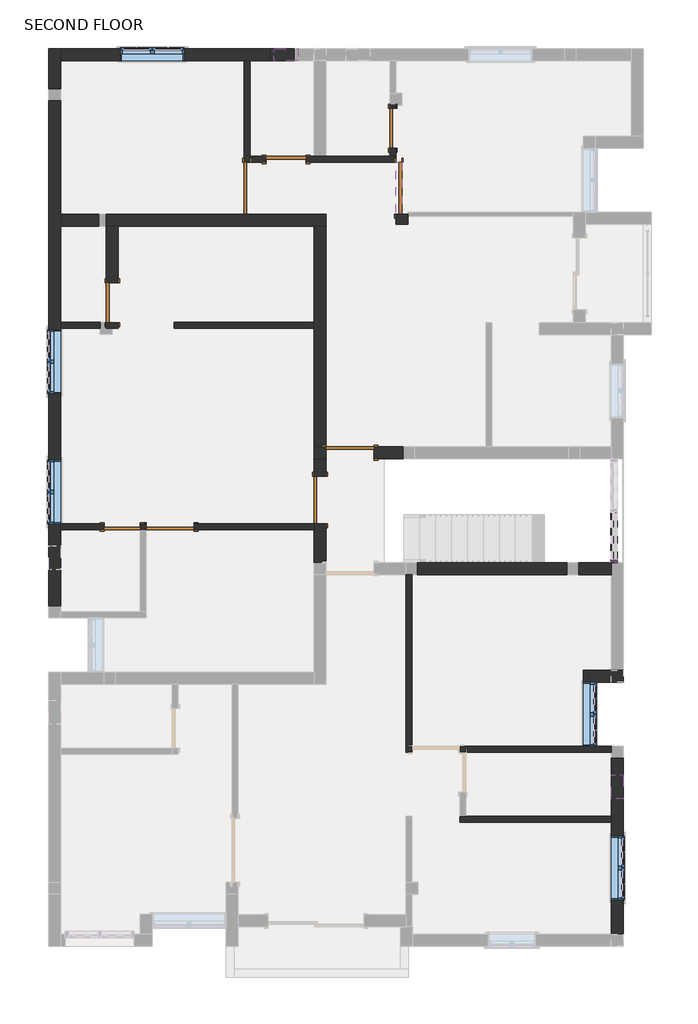
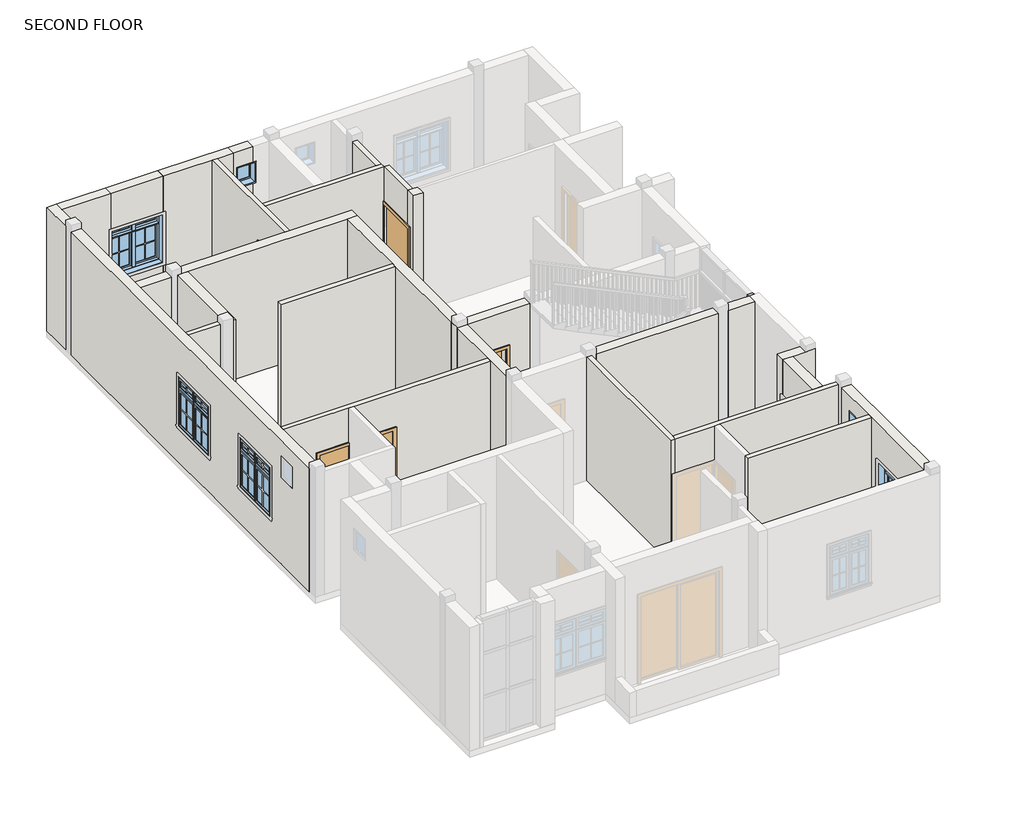
# One storey, part 2 of 6: 29 walls, 9 doors, 7 windows, 3 members.
"""IFC4 building model written with IfcOpenShell, lengths in millimetres."""

from ifc_helpers import new_model, si_unit, frame, origin, place, context, project, spatial, polyline, outline, extrude, faceted_brep, transform, mapped, element, save
from components import door_64f31108, door_78caadf7, door_214872d5, door_bb98abfd, door_43e5c869, door_0217d254, single_flush_3_x7_a90ba1ad, single_flush_3_x7_e5f9f3c4, member_f1f71bde, member_00c01c4d, member_ecafcbb3, window_abb441dd, window_casement_double_awning_double_4_x4_dd9041c6

model = new_model("IFC4")

# Units and contexts
model_context = context("Model", 3, world=origin())
ifc_project = project(units=[si_unit("LENGTHUNIT", "METRE", prefix="MILLI")], contexts=[model_context])

# Site, building, storey
site = spatial("IfcSite", under=ifc_project)
building = spatial("IfcBuilding", under=site)
storey = spatial("IfcBuildingStorey", under=building, Name="SECOND FLOOR", Elevation=6400.8)

# Doors
placement = place(None, origin())
door_shape = door_64f31108(model_context)
element("IfcDoor", 1, ObjectType="Single-Flush : 2'3\"X7'", at=placement, inside=storey, context=model_context, shape_type="MappedRepresentation", body=[
    mapped(door_shape, transform((-5358.7865981, 175.2287587, 6400.8), x_axis=(1.0, 0.0, 0.0), y_axis=(0.0, 1.0, 0.0), z_axis=(0.0, 0.0, 1.0))),
])
door_2_shape = door_78caadf7(model_context)
element("IfcDoor", 2, ObjectType="Single-Flush : 2'6\"X7'", at=placement, inside=storey, context=model_context, shape_type="MappedRepresentation", body=[
    mapped(door_2_shape, transform((-196.2365981, 7776.1787587, 6400.8), x_axis=(0.0, -1.0, 0.0), y_axis=(1.0, 0.0, 0.0), z_axis=(0.0, 0.0, 1.0))),
])
door_3_shape = door_214872d5(model_context)
element("IfcDoor", 3, ObjectType="Single-Flush : 2'6\"X7'", at=placement, inside=storey, context=model_context, shape_type="MappedRepresentation", body=[
    mapped(door_3_shape, transform((-2234.5865981, 7185.6287587, 6400.8), x_axis=(1.0, 0.0, 0.0), y_axis=(0.0, 1.0, 0.0), z_axis=(0.0, 0.0, 1.0))),
])
door_4_shape = door_bb98abfd(model_context)
element("IfcDoor", 4, ObjectType="Single-Flush : 2'6\"X7'", at=placement, inside=storey, context=model_context, shape_type="MappedRepresentation", body=[
    mapped(door_4_shape, transform((-5549.2865981, 4455.1287587, 6400.8), x_axis=(0.0, 1.0, 0.0), y_axis=(-1.0, 0.0, 0.0), z_axis=(0.0, 0.0, 1.0))),
])
door_5_shape = door_43e5c869(model_context)
element("IfcDoor", 5, ObjectType="Single-Flush : 3'3\"X7'", at=placement, inside=storey, context=model_context, shape_type="MappedRepresentation", body=[
    mapped(door_5_shape, transform((-2977.5365981, 6633.1787587, 6400.8), x_axis=(0.0, -1.0, 0.0), y_axis=(1.0, 0.0, 0.0), z_axis=(0.0, 0.0, 1.0))),
])
door_6_shape = door_0217d254(model_context)
element("IfcDoor", 6, ObjectType="Single-Flush : 3'3\"X7'", at=placement, inside=storey, context=model_context, shape_type="MappedRepresentation", body=[
    mapped(door_6_shape, transform((-81.9365981, 6633.1787587, 6400.8), x_axis=(0.0, -1.0, 0.0), y_axis=(1.0, 0.0, 0.0), z_axis=(0.0, 0.0, 1.0))),
])
single_flush_3_x7_shape = single_flush_3_x7_a90ba1ad(model_context)
element("IfcDoor", 7, ObjectType="Single-Flush : 3'X7'", at=placement, inside=storey, context=model_context, shape_type="MappedRepresentation", body=[
    mapped(single_flush_3_x7_shape, transform((-1586.8865981, 689.5787587, 6400.8), x_axis=(0.0, -1.0, 0.0), y_axis=(1.0, 0.0, 0.0), z_axis=(0.0, 0.0, 1.0))),
])
element("IfcDoor", 8, ObjectType="Single-Flush : 3'X7'", at=placement, inside=storey, context=model_context, shape_type="MappedRepresentation", body=[
    mapped(single_flush_3_x7_shape, transform((-1015.3865981, 1591.2787587, 6400.8), x_axis=(-1.0, 0.0, 0.0), y_axis=(0.0, -1.0, 0.0), z_axis=(0.0, 0.0, 1.0))),
])
single_flush_3_x7_2_shape = single_flush_3_x7_e5f9f3c4(model_context)
element("IfcDoor", 9, ObjectType="Single-Flush : 3'X7'", at=placement, inside=storey, context=model_context, shape_type="MappedRepresentation", body=[
    mapped(single_flush_3_x7_2_shape, transform((-4444.3865981, 175.2287587, 6400.8), x_axis=(-1.0, 0.0, 0.0), y_axis=(0.0, -1.0, 0.0), z_axis=(0.0, 0.0, 1.0))),
])

# Members
member_shape = member_f1f71bde(model_context)
element("IfcMember", 10, ObjectType="Rectangular Mullion : 2.5\" x 5\" rectangular", at=placement, inside=storey, context=model_context, shape_type="MappedRepresentation", body=[
    mapped(member_shape, transform((4026.5134019, -440.7212413, 6400.8), x_axis=(0.0, 0.0, -1.0), y_axis=(1.0, 0.0, 0.0), z_axis=(0.0, -1.0, 0.0))),
])
member_2_shape = member_00c01c4d(model_context)
element("IfcMember", 11, ObjectType="Rectangular Mullion : 2.5\" x 5\" rectangular", at=placement, inside=storey, context=model_context, shape_type="MappedRepresentation", body=[
    mapped(member_2_shape, transform((4026.5134019, -504.2212413, 7956.55), x_axis=(0.0, -1.0, 0.0), y_axis=(1.0, 0.0, 0.0), z_axis=(0.0, 0.0, 1.0))),
])
member_3_shape = member_ecafcbb3(model_context)
element("IfcMember", 12, ObjectType="Rectangular Mullion : 2.5\" x 5\" rectangular", at=placement, inside=storey, context=model_context, shape_type="MappedRepresentation", body=[
    mapped(member_3_shape, transform((4026.5134019, -504.2212413, 9448.8), x_axis=(0.0, -1.0, 0.0), y_axis=(1.0, 0.0, 0.0), z_axis=(0.0, 0.0, 1.0))),
])

# Walls
element("IfcWall", 13, ObjectType="4.5\"", at=placement, inside=storey, context=model_context, shape_type="Brep", body=[
    faceted_brep([(-3034.6865981, 6137.8787587, 9448.8), (-3034.6865981, 9071.5787587, 9448.8), (-3034.6865981, 9071.5787587, 6400.8), (-3034.6865981, 7128.4787587, 6400.8), (-3034.6865981, 7128.4787587, 8534.4), (-3034.6865981, 6137.8787587, 8534.4), (-2920.3865981, 9071.5787587, 9448.8), (-2920.3865981, 7242.7787587, 9448.8), (-2920.3865981, 7128.4787587, 9448.8), (-2920.3865981, 6137.8787587, 9448.8), (-2920.3865981, 6137.8787587, 8534.4), (-2920.3865981, 7128.4787587, 8534.4), (-2920.3865981, 7128.4787587, 6400.8), (-2920.3865981, 7242.7787587, 6400.8), (-2920.3865981, 9071.5787587, 6400.8)], [[[0, 1, 2, 3, 4, 5]], [[6, 7, 8, 9, 10, 11, 12, 13, 14]], [[2, 14, 13, 12, 3]], [[1, 0, 9, 8, 7, 6]], [[2, 1, 6, 14]], [[9, 0, 5, 10]], [[4, 11, 10, 5]], [[11, 4, 3, 12]]]),
])
element("IfcWall", 14, ObjectType="4.5\"", at=placement, inside=storey, context=model_context, shape_type="Brep", body=[
    faceted_brep([(-1853.5865981, 7128.4787587, 8534.4), (-1853.5865981, 7128.4787587, 6400.8), (-139.0865981, 7128.4787587, 6400.8), (-139.0865981, 7128.4787587, 9448.8), (-2920.3865981, 7128.4787587, 9448.8), (-2920.3865981, 7128.4787587, 8534.4), (-2920.3865981, 7128.4787587, 6400.8), (-2615.5865981, 7128.4787587, 6400.8), (-2615.5865981, 7128.4787587, 8534.4), (-139.0865981, 7242.7787587, 6400.8), (-253.3865981, 7242.7787587, 6400.8), (-1472.5865981, 7242.7787587, 6400.8), (-1701.1865981, 7242.7787587, 6400.8), (-1853.5865981, 7242.7787587, 6400.8), (-1853.5865981, 7242.7787587, 8534.4), (-2615.5865981, 7242.7787587, 8534.4), (-2615.5865981, 7242.7787587, 6400.8), (-2920.3865981, 7242.7787587, 6400.8), (-2920.3865981, 7242.7787587, 9448.8), (-1701.1865981, 7242.7787587, 9448.8), (-1472.5865981, 7242.7787587, 9448.8), (-253.3865981, 7242.7787587, 9448.8), (-139.0865981, 7242.7787587, 9448.8)], [[[0, 1, 2, 3, 4, 5, 6, 7, 8]], [[9, 10, 11, 12, 13, 14, 15, 16, 17, 18, 19, 20, 21, 22]], [[7, 6, 17, 16]], [[2, 1, 13, 12, 11, 10, 9]], [[4, 3, 22, 21, 20, 19, 18]], [[6, 5, 4, 18, 17]], [[3, 2, 9, 22]], [[14, 13, 1, 0]], [[15, 14, 0, 8]], [[16, 15, 8, 7]]]),
])
element("IfcWall", 15, ObjectType="4.5\"", at=placement, inside=storey, context=model_context, shape_type="SweptSolid", body=[
    extrude(outline(polyline([(7395.1787587, 8534.4), (7395.1787587, 6400.8), (7242.7787587, 6400.8), (7242.7787587, 9448.8), (8214.4921256, 9448.8), (8214.4921256, 6400.8), (8157.1787587, 6400.8), (8157.1787587, 8534.4), (7395.1787587, 8534.4)])), frame((-253.3865981, 0.0, 0.0), z_axis=(1.0, 0.0, 0.0), x_axis=(0.0, 1.0, 0.0)), (0.0, 0.0, 1.0), 114.3),
])
element("IfcWall", 16, ObjectType="4.5\"", at=placement, inside=storey, context=model_context, shape_type="SweptSolid", body=[
    extrude(outline(polyline([(-4368.1865981, 4080.4787587), (-1701.1865981, 4080.4787587), (-1701.1865981, 3966.1787587), (-4368.1865981, 3966.1787587), (-4368.1865981, 4080.4787587)])), frame((0.0, 0.0, 6400.8), z_axis=(0.0, 0.0, 1.0), x_axis=(1.0, 0.0, 0.0)), (0.0, 0.0, 1.0), 3048.0),
])
element("IfcWall", 17, ObjectType="4.5\"", at=placement, inside=storey, context=model_context, shape_type="SweptSolid", body=[
    extrude(outline(polyline([(-5786.6284021, 3966.1787587), (-6539.8865981, 3966.1787587), (-6539.8865981, 4080.4787587), (-5786.6284021, 4080.4787587), (-5786.6284021, 3966.1787587)])), frame((0.0, 0.0, 6400.8), z_axis=(0.0, 0.0, 1.0), x_axis=(1.0, 0.0, 0.0)), (0.0, 0.0, 1.0), 3048.0),
])
element("IfcWall", 18, ObjectType="4.5\"", at=placement, inside=storey, context=model_context, shape_type="Brep", body=[
    faceted_brep([(-5663.5865981, 4080.4787587, 9448.8), (-5558.0284021, 4080.4787587, 9448.8), (-5434.9865981, 4080.4787587, 9448.8), (-5434.9865981, 4080.4787587, 8534.4), (-5558.0284021, 4080.4787587, 8534.4), (-5663.5865981, 4080.4787587, 8534.4), (-5663.5865981, 3966.1787587, 6400.8), (-5558.0284021, 3966.1787587, 6400.8), (-5434.9865981, 3966.1787587, 6400.8), (-5434.9865981, 3966.1787587, 9448.8), (-5558.0284021, 3966.1787587, 9448.8), (-5663.5865981, 3966.1787587, 9448.8), (-5663.5865981, 4074.1287587, 6400.8), (-5558.0284021, 4074.1287587, 6400.8), (-5434.9865981, 4074.1287587, 6400.8), (-5434.9865981, 4074.1287587, 8534.4), (-5558.0284021, 4074.1287587, 8534.4), (-5663.5865981, 4074.1287587, 8534.4)], [[[0, 1, 2, 3, 4, 5]], [[6, 7, 8, 9, 10, 11]], [[8, 7, 6, 12, 13, 14]], [[2, 1, 0, 11, 10, 9]], [[9, 8, 14, 15, 3, 2]], [[15, 16, 17, 5, 4, 3]], [[17, 16, 15, 14, 13, 12]], [[6, 11, 0, 5, 17, 12]]]),
])
element("IfcWall", 19, ObjectType="4.5\"", at=placement, inside=storey, context=model_context, shape_type="Brep", body=[
    faceted_brep([(-4901.5865981, 232.3787587, 6400.8), (-5015.8865981, 232.3787587, 6400.8), (-5015.8865981, 232.3787587, 8534.4), (-5701.6865981, 232.3787587, 8534.4), (-5701.6865981, 232.3787587, 6400.8), (-6539.8865981, 232.3787587, 6400.8), (-6539.8865981, 232.3787587, 7315.2), (-6539.8865981, 232.3787587, 8534.4), (-6539.8865981, 232.3787587, 9448.8), (-1701.1865981, 232.3787587, 9448.8), (-1701.1865981, 232.3787587, 8534.4), (-1701.1865981, 232.3787587, 6400.8), (-3987.1865981, 232.3787587, 6400.8), (-3987.1865981, 232.3787587, 8534.4), (-4901.5865981, 232.3787587, 8534.4), (-5015.8865981, 118.0787587, 8534.4), (-5015.8865981, 118.0787587, 6400.8), (-4901.5865981, 118.0787587, 6400.8), (-4901.5865981, 118.0787587, 8534.4), (-3987.1865981, 118.0787587, 8534.4), (-3987.1865981, 118.0787587, 6400.8), (-1701.1865981, 118.0787587, 6400.8), (-1701.1865981, 118.0787587, 9448.8), (-4901.5865981, 118.0787587, 9448.8), (-5015.8865981, 118.0787587, 9448.8), (-6539.8865981, 118.0787587, 9448.8), (-6539.8865981, 118.0787587, 6400.8), (-5701.6865981, 118.0787587, 6400.8), (-5701.6865981, 118.0787587, 8534.4)], [[[0, 1, 2, 3, 4, 5, 6, 7, 8, 9, 10, 11, 12, 13, 14]], [[15, 16, 17, 18, 19, 20, 21, 22, 23, 24, 25, 26, 27, 28]], [[12, 11, 21, 20]], [[27, 26, 5, 4]], [[17, 16, 1, 0]], [[9, 8, 25, 24, 23, 22]], [[8, 7, 6, 5, 26, 25]], [[11, 10, 9, 22, 21]], [[18, 17, 0, 14]], [[19, 18, 14, 13]], [[20, 19, 13, 12]], [[2, 1, 16, 15]], [[3, 2, 15, 28]], [[4, 3, 28, 27]]]),
])
element("IfcWall", 20, ObjectType="4.5\"", at=placement, inside=storey, context=model_context, shape_type="Brep", body=[
    faceted_brep([(51.4134019, -732.8212413, 6400.8), (51.4134019, -4123.7212413, 6400.8), (51.4134019, -4123.7212413, 9448.8), (51.4134019, -732.8212413, 9448.8), (165.7134019, -732.8212413, 6400.8), (165.7134019, -732.8212413, 9448.8), (165.7134019, -4009.4212413, 9448.8), (165.7134019, -4123.7212413, 9448.8), (165.7134019, -4123.7212413, 8534.4), (165.7134019, -4123.7212413, 6400.8)], [[[0, 1, 2, 3]], [[4, 5, 6, 7, 8, 9]], [[1, 0, 4, 9]], [[3, 2, 7, 6, 5]], [[0, 3, 5, 4]], [[2, 1, 9, 8, 7]]]),
])
element("IfcWall", 21, ObjectType="4.5\"", at=placement, inside=storey, context=model_context, shape_type="Brep", body=[
    faceted_brep([(3975.7134019, -4123.7212413, 6400.8), (3975.7134019, -4123.7212413, 9448.8), (1194.4134019, -4123.7212413, 9448.8), (1080.1134019, -4123.7212413, 9448.8), (165.7134019, -4123.7212413, 9448.8), (165.7134019, -4123.7212413, 8534.4), (1080.1134019, -4123.7212413, 8534.4), (1080.1134019, -4123.7212413, 6400.8), (1194.4134019, -4123.7212413, 6400.8), (3975.7134019, -4009.4212413, 9448.8), (3975.7134019, -4009.4212413, 6400.8), (3670.9134019, -4009.4212413, 6400.8), (3442.3134019, -4009.4212413, 6400.8), (1080.1134019, -4009.4212413, 6400.8), (1080.1134019, -4009.4212413, 8534.4), (165.7134019, -4009.4212413, 8534.4), (165.7134019, -4009.4212413, 9448.8), (3442.3134019, -4009.4212413, 9448.8), (3670.9134019, -4009.4212413, 9448.8)], [[[0, 1, 2, 3, 4, 5, 6, 7, 8]], [[9, 10, 11, 12, 13, 14, 15, 16, 17, 18]], [[10, 0, 8, 7, 13, 12, 11]], [[1, 0, 10, 9]], [[4, 3, 2, 1, 9, 18, 17, 16]], [[4, 16, 15, 5]], [[14, 6, 5, 15]], [[6, 14, 13, 7]]]),
])
element("IfcWall", 22, ObjectType="4.5\"", at=placement, inside=storey, context=model_context, shape_type="Brep", body=[
    faceted_brep([(3975.7134019, -5342.9212413, 6400.8), (1194.4134019, -5342.9212413, 6400.8), (1080.1134019, -5342.9212413, 6400.8), (1080.1134019, -5342.9212413, 9448.8), (1194.4134019, -5342.9212413, 9448.8), (3975.7134019, -5342.9212413, 9448.8), (3975.7134019, -5457.2212413, 6400.8), (3975.7134019, -5457.2212413, 9448.8), (1080.1134019, -5457.2212413, 9448.8), (1080.1134019, -5457.2212413, 6400.8)], [[[0, 1, 2, 3, 4, 5]], [[6, 7, 8, 9]], [[2, 1, 0, 6, 9]], [[5, 4, 3, 8, 7]], [[0, 5, 7, 6]], [[3, 2, 9, 8]]]),
])
element("IfcWall", 23, ObjectType="4.5\"", at=placement, inside=storey, context=model_context, shape_type="SweptSolid", body=[
    extrude(outline(polyline([(-139.0865981, 6175.9787587), (-139.0865981, 7128.4787587), (-24.7865981, 7128.4787587), (-24.7865981, 6175.9787587), (-139.0865981, 6175.9787587)])), frame((0.0, 0.0, 8534.4), z_axis=(0.0, 0.0, 1.0), x_axis=(1.0, 0.0, 0.0)), (0.0, 0.0, 1.0), 914.4),
])
element("IfcWall", 24, ObjectType="9\"", at=placement, inside=storey, context=model_context, shape_type="Brep", body=[
    faceted_brep([(-6768.4865981, 9300.1787587, 6400.8), (-6768.4865981, 8531.2343988, 6400.8), (-6768.4865981, 8531.2343988, 9448.8), (-6768.4865981, 9300.1787587, 9448.8), (-6539.8865981, 9300.1787587, 6400.8), (-6539.8865981, 9300.1787587, 9448.8), (-6539.8865981, 9071.5787587, 9448.8), (-6539.8865981, 8531.2343988, 9448.8), (-6539.8865981, 8531.2343988, 6400.8), (-6539.8865981, 9071.5787587, 6400.8)], [[[0, 1, 2, 3]], [[4, 5, 6, 7, 8, 9]], [[1, 0, 4, 9, 8]], [[2, 1, 8, 7]], [[3, 2, 7, 6, 5]], [[0, 3, 5, 4]]]),
])
element("IfcWall", 25, ObjectType="9\"", at=placement, inside=storey, context=model_context, shape_type="Brep", body=[
    faceted_brep([(-6768.4865981, 8302.6343988, 6400.8), (-6768.4865981, -1329.7212413, 6400.8), (-6768.4865981, -1329.7212413, 9448.8), (-6768.4865981, 8302.6343988, 9448.8), (-6768.4865981, 1451.5787587, 8534.4), (-6768.4865981, 232.3787587, 8534.4), (-6768.4865981, 232.3787587, 7315.2), (-6768.4865981, 1451.5787587, 7315.2), (-6768.4865981, 3937.3572861, 8534.4), (-6768.4865981, 2718.1572861, 8534.4), (-6768.4865981, 2718.1572861, 7315.2), (-6768.4865981, 3937.3572861, 7315.2), (-6768.4865981, -186.7212413, 9067.8), (-6768.4865981, -643.9212413, 9067.8), (-6768.4865981, -643.9212413, 8534.4), (-6768.4865981, -186.7212413, 8534.4), (-6539.8865981, 8302.6343988, 6400.8), (-6539.8865981, 8302.6343988, 9448.8), (-6539.8865981, 6137.8787587, 9448.8), (-6539.8865981, 5909.2787587, 9448.8), (-6539.8865981, 4080.4787587, 9448.8), (-6539.8865981, 3966.1787587, 9448.8), (-6539.8865981, 232.3787587, 9448.8), (-6539.8865981, 118.0787587, 9448.8), (-6539.8865981, -1329.7212413, 9448.8), (-6539.8865981, -1329.7212413, 6400.8), (-6539.8865981, 118.0787587, 6400.8), (-6539.8865981, 232.3787587, 6400.8), (-6539.8865981, 3966.1787587, 6400.8), (-6539.8865981, 4080.4787587, 6400.8), (-6539.8865981, 5909.2787587, 6400.8), (-6539.8865981, 6137.8787587, 6400.8), (-6539.8865981, 1451.5787587, 8534.4), (-6539.8865981, 1451.5787587, 7315.2), (-6539.8865981, 232.3787587, 7315.2), (-6539.8865981, 232.3787587, 8534.4), (-6539.8865981, 3937.3572861, 8534.4), (-6539.8865981, 3937.3572861, 7315.2), (-6539.8865981, 2718.1572861, 7315.2), (-6539.8865981, 2718.1572861, 8534.4), (-6539.8865981, -186.7212413, 9067.8), (-6539.8865981, -186.7212413, 8534.4), (-6539.8865981, -643.9212413, 8534.4), (-6539.8865981, -643.9212413, 9067.8)], [[[0, 1, 2, 3], [4, 5, 6, 7], [8, 9, 10, 11], [12, 13, 14, 15]], [[16, 17, 18, 19, 20, 21, 22, 23, 24, 25, 26, 27, 28, 29, 30, 31], [32, 33, 34, 35], [36, 37, 38, 39], [40, 41, 42, 43]], [[1, 0, 16, 31, 30, 29, 28, 27, 26, 25]], [[2, 1, 25, 24]], [[3, 2, 24, 23, 22, 21, 20, 19, 18, 17]], [[0, 3, 17, 16]], [[33, 32, 4, 7]], [[34, 33, 7, 6]], [[35, 34, 6, 5]], [[32, 35, 5, 4]], [[37, 36, 8, 11]], [[38, 37, 11, 10]], [[39, 38, 10, 9]], [[36, 39, 9, 8]], [[41, 40, 12, 15]], [[42, 41, 15, 14]], [[43, 42, 14, 13]], [[40, 43, 13, 12]]]),
])
element("IfcWall", 26, ObjectType="9\"", at=placement, inside=storey, context=model_context, shape_type="Brep", body=[
    faceted_brep([(4204.3134019, -7590.8212413, 6400.8), (4204.3134019, -4238.0212413, 6400.8), (4204.3134019, -4238.0212413, 9448.8), (4204.3134019, -7590.8212413, 9448.8), (4204.3134019, -6938.5380734, 8534.4), (4204.3134019, -5719.3380734, 8534.4), (4204.3134019, -5719.3380734, 7315.2), (4204.3134019, -6938.5380734, 7315.2), (4204.3134019, -5004.2995612, 9067.8), (4204.3134019, -4547.0995612, 9067.8), (4204.3134019, -4547.0995612, 8534.4), (4204.3134019, -5004.2995612, 8534.4), (3975.7134019, -7590.8212413, 6400.8), (3975.7134019, -7590.8212413, 9448.8), (3975.7134019, -5457.2212413, 9448.8), (3975.7134019, -5342.9212413, 9448.8), (3975.7134019, -4238.0212413, 9448.8), (3975.7134019, -4238.0212413, 6400.8), (3975.7134019, -5342.9212413, 6400.8), (3975.7134019, -5457.2212413, 6400.8), (3975.7134019, -6938.5380734, 8534.4), (3975.7134019, -6938.5380734, 7315.2), (3975.7134019, -5719.3380734, 7315.2), (3975.7134019, -5719.3380734, 8534.4), (3975.7134019, -5004.2995612, 9067.8), (3975.7134019, -5004.2995612, 8534.4), (3975.7134019, -4547.0995612, 8534.4), (3975.7134019, -4547.0995612, 9067.8)], [[[0, 1, 2, 3], [4, 5, 6, 7], [8, 9, 10, 11]], [[12, 13, 14, 15, 16, 17, 18, 19], [20, 21, 22, 23], [24, 25, 26, 27]], [[1, 0, 12, 19, 18, 17]], [[2, 1, 17, 16]], [[3, 2, 16, 15, 14, 13]], [[0, 3, 13, 12]], [[21, 20, 4, 7]], [[22, 21, 7, 6]], [[23, 22, 6, 5]], [[20, 23, 5, 4]], [[25, 24, 8, 11]], [[26, 25, 11, 10]], [[27, 26, 10, 9]], [[24, 27, 9, 8]]]),
])
element("IfcWall", 27, ObjectType="9\"", at=placement, inside=storey, context=model_context, shape_type="SweptSolid", body=[
    extrude(outline(polyline([(3670.9134019, -2790.2212413), (3670.9134019, -4009.4212413), (3442.3134019, -4009.4212413), (3442.3134019, -2790.2212413), (3670.9134019, -2790.2212413)])), frame((0.0, 0.0, 6400.8), z_axis=(0.0, 0.0, 1.0), x_axis=(1.0, 0.0, 0.0)), (0.0, 0.0, 1.0), 914.4),
    extrude(outline(polyline([(3670.9134019, -2790.2212413), (3670.9134019, -4009.4212413), (3442.3134019, -4009.4212413), (3442.3134019, -2790.2212413), (3670.9134019, -2790.2212413)])), frame((0.0, 0.0, 8534.4), z_axis=(0.0, 0.0, 1.0), x_axis=(1.0, 0.0, 0.0)), (0.0, 0.0, 1.0), 914.4),
])
element("IfcWall", 28, ObjectType="9\"", at=placement, inside=storey, context=model_context, shape_type="Brep", body=[
    faceted_brep([(3442.3134019, -2790.2212413, 6400.8), (3670.9134019, -2790.2212413, 6400.8), (4204.3134019, -2790.2212413, 6400.8), (4204.3134019, -2790.2212413, 9448.8), (3975.7134019, -2790.2212413, 9448.8), (3670.9134019, -2790.2212413, 9448.8), (3442.3134019, -2790.2212413, 9448.8), (3442.3134019, -2790.2212413, 8534.4), (3442.3134019, -2790.2212413, 7315.2), (3442.3134019, -2561.6212413, 6400.8), (3442.3134019, -2561.6212413, 9448.8), (3975.7134019, -2561.6212413, 9448.8), (4204.3134019, -2561.6212413, 9448.8), (4204.3134019, -2561.6212413, 6400.8), (3975.7134019, -2561.6212413, 6400.8)], [[[0, 1, 2, 3, 4, 5, 6, 7, 8]], [[9, 10, 11, 12, 13, 14]], [[2, 1, 0, 9, 14, 13]], [[6, 5, 4, 3, 12, 11, 10]], [[0, 8, 7, 6, 10, 9]], [[3, 2, 13, 12]]]),
])
element("IfcWall", 29, ObjectType="9\"", at=placement, inside=storey, context=model_context, shape_type="SweptSolid", body=[
    extrude(outline(polyline([(3352.7127672, -504.2212413), (3975.7134019, -504.2212413), (3975.7134019, -732.8212413), (3352.7127672, -732.8212413), (3352.7127672, -504.2212413)])), frame((0.0, 0.0, 6400.8), z_axis=(0.0, 0.0, 1.0), x_axis=(1.0, 0.0, 0.0)), (0.0, 0.0, 1.0), 3048.0),
])
element("IfcWall", 30, ObjectType="9\"", at=placement, inside=storey, context=model_context, shape_type="SweptSolid", body=[
    extrude(outline(polyline([(269.7035962, -504.2212413), (3124.1127672, -504.2212413), (3124.1127672, -732.8212413), (269.7035962, -732.8212413), (269.7035962, -504.2212413)])), frame((0.0, 0.0, 6400.8), z_axis=(0.0, 0.0, 1.0), x_axis=(1.0, 0.0, 0.0)), (0.0, 0.0, 1.0), 3048.0),
])
element("IfcWall", 31, ObjectType="9\"", at=placement, inside=storey, context=model_context, shape_type="Brep", body=[
    faceted_brep([(-1472.5865981, 1705.5787587, 8534.4), (-1472.5865981, 1705.5787587, 6400.8), (-1701.1865981, 1705.5787587, 6400.8), (-1701.1865981, 1705.5787587, 9448.8), (-1472.5865981, 1705.5787587, 9448.8), (0.651657, 1705.5787587, 9448.8), (0.651657, 1705.5787587, 6400.8), (-558.1865981, 1705.5787587, 6400.8), (-558.1865981, 1705.5787587, 8534.4), (-1701.1865981, 1476.9787587, 6400.8), (-1472.5865981, 1476.9787587, 6400.8), (-1472.5865981, 1476.9787587, 8534.4), (-558.1865981, 1476.9787587, 8534.4), (-558.1865981, 1476.9787587, 6400.8), (0.651657, 1476.9787587, 6400.8), (0.651657, 1476.9787587, 9448.8), (-1472.5865981, 1476.9787587, 9448.8), (-1701.1865981, 1476.9787587, 9448.8), (-1701.1865981, 1693.0966521, 9448.8)], [[[0, 1, 2, 3, 4, 5, 6, 7, 8]], [[9, 10, 11, 12, 13, 14, 15, 16, 17]], [[7, 6, 14, 13]], [[2, 1, 10, 9]], [[5, 4, 3, 18, 17, 16, 15]], [[6, 5, 15, 14]], [[3, 2, 9, 17, 18]], [[11, 10, 1, 0]], [[12, 11, 0, 8]], [[13, 12, 8, 7]]]),
])
element("IfcWall", 32, ObjectType="9\"", at=placement, inside=storey, context=model_context, shape_type="Brep", body=[
    faceted_brep([(-2539.3865981, 9300.1787587, 6400.8), (-4177.6865981, 9300.1787587, 6400.8), (-4177.6865981, 9300.1787587, 7315.2), (-4177.6865981, 9300.1787587, 8534.4), (-4177.6865981, 9300.1787587, 9448.8), (-2539.3865981, 9300.1787587, 9448.8), (-2539.3865981, 9071.5787587, 6400.8), (-2539.3865981, 9071.5787587, 9448.8), (-2920.3865981, 9071.5787587, 9448.8), (-3034.6865981, 9071.5787587, 9448.8), (-4177.6865981, 9071.5787587, 9448.8), (-4177.6865981, 9071.5787587, 8534.4), (-4177.6865981, 9071.5787587, 7315.2), (-4177.6865981, 9071.5787587, 6400.8), (-3034.6865981, 9071.5787587, 6400.8), (-2920.3865981, 9071.5787587, 6400.8)], [[[0, 1, 2, 3, 4, 5]], [[6, 7, 8, 9, 10, 11, 12, 13, 14, 15]], [[1, 0, 6, 15, 14, 13]], [[4, 3, 2, 1, 13, 12, 11, 10]], [[5, 4, 10, 9, 8, 7]], [[0, 5, 7, 6]]]),
])
element("IfcWall", 33, ObjectType="9\"", at=placement, inside=storey, context=model_context, shape_type="Brep", body=[
    faceted_brep([(-5396.8865981, 9300.1787587, 6400.8), (-6539.8865981, 9300.1787587, 6400.8), (-6539.8865981, 9300.1787587, 9448.8), (-5396.8865981, 9300.1787587, 9448.8), (-5396.8865981, 9300.1787587, 8534.4), (-5396.8865981, 9300.1787587, 7315.2), (-5396.8865981, 9071.5787587, 6400.8), (-5396.8865981, 9071.5787587, 7315.2), (-5396.8865981, 9071.5787587, 8534.4), (-5396.8865981, 9071.5787587, 9448.8), (-6539.8865981, 9071.5787587, 9448.8), (-6539.8865981, 9071.5787587, 6400.8)], [[[0, 1, 2, 3, 4, 5]], [[6, 7, 8, 9, 10, 11]], [[1, 0, 6, 11]], [[3, 2, 10, 9]], [[0, 5, 4, 3, 9, 8, 7, 6]], [[2, 1, 11, 10]]]),
])
element("IfcWall", 34, ObjectType="9\"", at=placement, inside=storey, context=model_context, shape_type="SweptSolid", body=[
    extrude(outline(polyline([(-5807.056564, 5909.2787587), (-6539.8865981, 5909.2787587), (-6539.8865981, 6137.8787587), (-5807.056564, 6137.8787587), (-5807.056564, 5909.2787587)])), frame((0.0, 0.0, 6400.8), z_axis=(0.0, 0.0, 1.0), x_axis=(1.0, 0.0, 0.0)), (0.0, 0.0, 1.0), 3048.0),
])
element("IfcWall", 35, ObjectType="9\"", at=placement, inside=storey, context=model_context, shape_type="Brep", body=[
    faceted_brep([(-5663.5865981, 5909.2787587, 6400.8), (-5434.9865981, 5909.2787587, 6400.8), (-1701.1865981, 5909.2787587, 6400.8), (-1472.5865981, 5909.2787587, 6400.8), (-1472.5865981, 5909.2787587, 9448.8), (-1701.1865981, 5909.2787587, 9448.8), (-5434.9865981, 5909.2787587, 9448.8), (-5578.456564, 5909.2787587, 9448.8), (-5663.5865981, 5909.2787587, 9448.8), (-5663.5865981, 6137.8787587, 6400.8), (-5663.5865981, 6137.8787587, 9448.8), (-5578.456564, 6137.8787587, 9448.8), (-3034.6865981, 6137.8787587, 9448.8), (-2920.3865981, 6137.8787587, 9448.8), (-1472.5865981, 6137.8787587, 9448.8), (-1472.5865981, 6137.8787587, 6400.8)], [[[0, 1, 2, 3, 4, 5, 6, 7, 8]], [[9, 10, 11, 12, 13, 14, 15]], [[3, 2, 1, 0, 9, 15]], [[8, 7, 6, 5, 4, 14, 13, 12, 11, 10]], [[4, 3, 15, 14]], [[0, 8, 10, 9]]]),
])
element("IfcWall", 36, ObjectType="9\"", at=placement, inside=storey, context=model_context, shape_type="Brep", body=[
    faceted_brep([(-1701.1865981, 5909.2787587, 6400.8), (-1701.1865981, 4080.4787587, 6400.8), (-1701.1865981, 3966.1787587, 6400.8), (-1701.1865981, 1705.5787587, 6400.8), (-1701.1865981, 1705.5787587, 9448.8), (-1701.1865981, 3966.1787587, 9448.8), (-1701.1865981, 4080.4787587, 9448.8), (-1701.1865981, 5909.2787587, 9448.8), (-1472.5865981, 5909.2787587, 6400.8), (-1472.5865981, 5909.2787587, 9448.8), (-1472.5865981, 1705.5787587, 9448.8), (-1472.5865981, 1705.5787587, 8534.4), (-1472.5865981, 1705.5787587, 6400.8)], [[[0, 1, 2, 3, 4, 5, 6, 7]], [[8, 9, 10, 11, 12]], [[3, 2, 1, 0, 8, 12]], [[7, 6, 5, 4, 10, 9]], [[0, 7, 9, 8]], [[4, 3, 12, 11, 10]]]),
])
element("IfcWall", 37, ObjectType="9\"", at=placement, inside=storey, context=model_context, shape_type="Brep", body=[
    faceted_brep([(-1701.1865981, 232.3787587, 8534.4), (-1701.1865981, 232.3787587, 6400.8), (-1701.1865981, 118.0787587, 6400.8), (-1701.1865981, -504.2212413, 6400.8), (-1701.1865981, -504.2212413, 9448.8), (-1701.1865981, 118.0787587, 9448.8), (-1701.1865981, 232.3787587, 9448.8), (-1701.1865981, 1464.4966521, 9448.8), (-1701.1865981, 1464.4966521, 6400.8), (-1701.1865981, 1146.7787587, 6400.8), (-1701.1865981, 1146.7787587, 8534.4), (-1472.5865981, -504.2212413, 6400.8), (-1472.5865981, 232.3787587, 6400.8), (-1472.5865981, 232.3787587, 8534.4), (-1472.5865981, 1146.7787587, 8534.4), (-1472.5865981, 1146.7787587, 6400.8), (-1472.5865981, 1464.4966521, 6400.8), (-1472.5865981, 1464.4966521, 9448.8), (-1472.5865981, -504.2212413, 9448.8), (-1472.5865981, -504.2212413, 8534.4)], [[[0, 1, 2, 3, 4, 5, 6, 7, 8, 9, 10]], [[11, 12, 13, 14, 15, 16, 17, 18, 19]], [[9, 8, 16, 15]], [[3, 2, 1, 12, 11]], [[7, 6, 5, 4, 18, 17]], [[8, 7, 17, 16]], [[4, 3, 11, 19, 18]], [[13, 12, 1, 0]], [[14, 13, 0, 10]], [[15, 14, 10, 9]]]),
])
element("IfcWall", 38, ObjectType="9\"", at=placement, inside=storey, context=model_context, shape_type="SweptSolid", body=[
    extrude(outline(polyline([(4080.4787587, 9448.8), (5909.2787587, 9448.8), (5909.2787587, 6400.8), (4836.1287587, 6400.8), (4836.1287587, 8534.4), (4080.4787587, 8534.4), (4080.4787587, 9448.8)])), frame((-5663.5865981, 0.0, 0.0), z_axis=(1.0, 0.0, 0.0), x_axis=(0.0, 1.0, 0.0)), (0.0, 0.0, 1.0), 228.6),
])
element("IfcWall", 39, ObjectType="9\"", at=placement, inside=storey, context=model_context, shape_type="SweptSolid", body=[
    extrude(outline(polyline([(-4177.6865981, 9071.5787587), (-5396.8865981, 9071.5787587), (-5396.8865981, 9300.1787587), (-4177.6865981, 9300.1787587), (-4177.6865981, 9071.5787587)])), frame((0.0, 0.0, 6400.8), z_axis=(0.0, 0.0, 1.0), x_axis=(1.0, 0.0, 0.0)), (0.0, 0.0, 1.0), 914.4),
    extrude(outline(polyline([(-4177.6865981, 9071.5787587), (-5396.8865981, 9071.5787587), (-5396.8865981, 9300.1787587), (-4177.6865981, 9300.1787587), (-4177.6865981, 9071.5787587)])), frame((0.0, 0.0, 8534.4), z_axis=(0.0, 0.0, 1.0), x_axis=(1.0, 0.0, 0.0)), (0.0, 0.0, 1.0), 914.4),
])
element("IfcWall", 40, ObjectType="9\"", at=placement, inside=storey, context=model_context, shape_type="SweptSolid", body=[
    extrude(outline(polyline([(6400.8, -2539.3865981), (6400.8, -2082.1865981), (8534.4, -2082.1865981), (8534.4, -2463.1865981), (9067.8, -2463.1865981), (9067.8, -2082.1865981), (9448.8, -2082.1865981), (9448.8, -2539.3865981), (6400.8, -2539.3865981)])), frame((0.0, 9071.5787587, 0.0), z_axis=(0.0, 1.0, 0.0), x_axis=(0.0, 0.0, 1.0)), (0.0, 0.0, 1.0), 228.6),
])
element("IfcWall", 41, ObjectType="9\"", at=placement, inside=storey, context=model_context, shape_type="Brep", body=[
    faceted_brep([(-139.0865981, 5947.3787587, 6400.8), (-139.0865981, 5947.3787587, 9448.8), (-139.0865981, 6175.9787587, 9448.8), (-139.0865981, 6175.9787587, 8534.4), (-139.0865981, 6137.8787587, 8534.4), (-139.0865981, 6137.8787587, 6400.8), (89.5134019, 5947.3787587, 9448.8), (89.5134019, 5947.3787587, 6400.8), (89.5134019, 6099.7787587, 6400.8), (89.5134019, 6137.8787587, 6400.8), (89.5134019, 6137.8787587, 8534.4), (89.5134019, 6175.9787587, 8534.4), (89.5134019, 6175.9787587, 9448.8), (89.5134019, 6099.7787587, 9448.8), (-24.7865981, 6175.9787587, 9448.8), (-24.7865981, 6175.9787587, 8534.4)], [[[0, 1, 2, 3, 4, 5]], [[6, 7, 8, 9, 10, 11, 12, 13]], [[7, 0, 5, 9, 8]], [[1, 0, 7, 6]], [[2, 1, 6, 13, 12, 14]], [[2, 14, 12, 11, 15, 3]], [[4, 10, 9, 5]], [[10, 4, 3, 15, 11]]]),
])

# Windows
window_shape = window_abb441dd(model_context)
element("IfcWindow", 42, ObjectType="Fixed : 1'6\"X1'9\"", at=placement, inside=storey, context=model_context, shape_type="MappedRepresentation", body=[
    mapped(window_shape, transform((-2196.4865981, 9185.8787587, 6400.8), x_axis=(1.0, 0.0, 0.0), y_axis=(0.0, 1.0, 0.0), z_axis=(0.0, 0.0, 1.0))),
])
element("IfcWindow", 43, ObjectType="Fixed : 1'6\"X1'9\"", at=placement, inside=storey, context=model_context, shape_type="MappedRepresentation", body=[
    mapped(window_shape, transform((4090.0134019, -4813.7995612, 6400.8), x_axis=(0.0, -1.0, 0.0), y_axis=(1.0, 0.0, 0.0), z_axis=(0.0, 0.0, 1.0))),
])
window_casement_double_awning_double_4_x4_shape = window_casement_double_awning_double_4_x4_dd9041c6(model_context)
element("IfcWindow", 44, ObjectType="Window-Casement-Double-Awning-Double : 4'X4'", at=placement, inside=storey, context=model_context, shape_type="MappedRepresentation", body=[
    mapped(window_casement_double_awning_double_4_x4_shape, transform((-4787.2865981, 9185.8787587, 6400.8), x_axis=(1.0, 0.0, 0.0), y_axis=(0.0, 1.0, 0.0), z_axis=(0.0, 0.0, 1.0))),
])
element("IfcWindow", 45, ObjectType="Window-Casement-Double-Awning-Double : 4'X4'", at=placement, inside=storey, context=model_context, shape_type="MappedRepresentation", body=[
    mapped(window_casement_double_awning_double_4_x4_shape, transform((3556.6134019, -3399.8212413, 6400.8), x_axis=(0.0, -1.0, 0.0), y_axis=(1.0, 0.0, 0.0), z_axis=(0.0, 0.0, 1.0))),
])
element("IfcWindow", 46, ObjectType="Window-Casement-Double-Awning-Double : 4'X4'", at=placement, inside=storey, context=model_context, shape_type="MappedRepresentation", body=[
    mapped(window_casement_double_awning_double_4_x4_shape, transform((4090.0134019, -6328.9380734, 6400.8), x_axis=(0.0, -1.0, 0.0), y_axis=(1.0, 0.0, 0.0), z_axis=(0.0, 0.0, 1.0))),
])
element("IfcWindow", 47, ObjectType="Window-Casement-Double-Awning-Double : 4'X4'", at=placement, inside=storey, context=model_context, shape_type="MappedRepresentation", body=[
    mapped(window_casement_double_awning_double_4_x4_shape, transform((-6654.1865981, 841.9787587, 6400.8), x_axis=(0.0, 1.0, 0.0), y_axis=(-1.0, 0.0, 0.0), z_axis=(0.0, 0.0, 1.0))),
])
element("IfcWindow", 48, ObjectType="Window-Casement-Double-Awning-Double : 4'X4'", at=placement, inside=storey, context=model_context, shape_type="MappedRepresentation", body=[
    mapped(window_casement_double_awning_double_4_x4_shape, transform((-6654.1865981, 3327.7572861, 6400.8), x_axis=(0.0, 1.0, 0.0), y_axis=(-1.0, 0.0, 0.0), z_axis=(0.0, 0.0, 1.0))),
])

save(model, "model.ifc")

# Revit data of these elements
# Type "Single-Flush : 2'3\"X7'"
#   Type Mark = "10"
#   Construction Type Id = "MDOOR"
#   Assembly Code = "C1020"
#   Analytic Construction = "Metal"
#   Thickness = 0' - 2"
#   Heat Transfer Coefficient (U) = 0.651978 BTU/(h·ft²·°F)
#   Height = 7' - 0"
#   Trim Projection Ext = 0' - 1"
#   Trim Projection Int = 0' - 1"
#   Trim Width = 0' - 3"
#   Width = 2' - 3"
#   Define Thermal Properties by = 1
#   Door Material = Door - Panel
#   Frame Material = Door - Frame
#   Visual Light Transmittance = 0
#   Solar Heat Gain Coefficient = 0
#   Function = (empty or 0)
#   Wall Closure = (empty or 0)
# Type "Single-Flush : 2'6\"X7'"
#   Type Mark = "9"
#   Construction Type Id = "MDOOR"
#   Assembly Code = "C1020"
#   Analytic Construction = "Metal"
#   Thickness = 0' - 2"
#   Heat Transfer Coefficient (U) = 0.651978 BTU/(h·ft²·°F)
#   Height = 7' - 0"
#   Trim Projection Ext = 0' - 1"
#   Trim Projection Int = 0' - 1"
#   Trim Width = 0' - 3"
#   Width = 2' - 6"
#   Define Thermal Properties by = 1
#   Door Material = Door - Panel
#   Frame Material = Door - Frame
#   Visual Light Transmittance = 0
#   Solar Heat Gain Coefficient = 0
#   Function = (empty or 0)
#   Wall Closure = (empty or 0)
# Type "Single-Flush : 3'3\"X7'"
#   Type Mark = "11"
#   Construction Type Id = "MDOOR"
#   Assembly Code = "C1020"
#   Analytic Construction = "Metal"
#   Thickness = 0' - 2"
#   Heat Transfer Coefficient (U) = 0.651978 BTU/(h·ft²·°F)
#   Height = 7' - 0"
#   Trim Projection Ext = 0' - 1"
#   Trim Projection Int = 0' - 1"
#   Trim Width = 0' - 3"
#   Width = 3' - 3"
#   Define Thermal Properties by = 1
#   Door Material = Door - Panel
#   Frame Material = Door - Frame
#   Visual Light Transmittance = 0
#   Solar Heat Gain Coefficient = 0
#   Function = (empty or 0)
#   Wall Closure = (empty or 0)
# Type "Single-Flush : 3'X7'"
#   Type Mark = "8"
#   Construction Type Id = "MDOOR"
#   Assembly Code = "C1020"
#   Analytic Construction = "Metal"
#   Thickness = 0' - 2"
#   Heat Transfer Coefficient (U) = 0.651978 BTU/(h·ft²·°F)
#   Height = 7' - 0"
#   Trim Projection Ext = 0' - 1"
#   Trim Projection Int = 0' - 1"
#   Trim Width = 0' - 3"
#   Width = 3' - 0"
#   Define Thermal Properties by = 1
#   Door Material = Door - Panel
#   Frame Material = Door - Frame
#   Visual Light Transmittance = 0
#   Solar Heat Gain Coefficient = 0
#   Function = (empty or 0)
#   Wall Closure = (empty or 0)
# Type "Rectangular Mullion : 2.5\" x 5\" rectangular"
#   built-in parameter 1007304 = 0.416667 (stored number, unit not read)
#   built-in parameter 1007301 = 0.104167 (stored number, unit not read)
#   built-in parameter 1007300 = 0.104167 (stored number, unit not read)
# Type "4.5\""
#   Assembly Code = "B2010"
#   Layers, outside or top first: 0' - 4 1/2" no material (function 1)
# Type "9\""
#   Assembly Code = "B2010"
#   Layers, outside or top first: 0' - 9" "wall" (function 1)
# Type "Fixed : 1'6\"X1'9\""
#   Type Mark = "24"
#   Construction Type Id = "GSP4R"
#   Assembly Code = "B2020100"
#   Analytic Construction = "1/8 in Pilkington single glazing"
#   Visual Light Transmittance = 0.9
#   Solar Heat Gain Coefficient = 0.78
#   Heat Transfer Coefficient (U) = 0.6496 BTU/(h·ft²·°F)
#   Height = 1' - 9"
#   Default Sill Height = 7' - 0"
#   Width = 1' - 6"
#   Window Inset = 0' - 0 3/4"
#   Define Thermal Properties by = 1
#   Glass Pane Material = Glass
#   Sash Material = Sash
#   Wall Closure = (empty or 0)
# Type "Window-Casement-Double-Awning-Double : 4'X4'"
#   Type Mark = "19"
#   Fire Rating = "0.5h"
#   Assembly Code = "B2020100"
#   Analytic Construction = "Double glazing - domestic"
#   Window Inset [instance default] = 0' - 0"
#   Wall Thickness [instance default] = 0' - 6"
#   Interior Wall Closure [instance default] = 0' - 2 1/4"
#   Half Width = 2' - 0"
#   Visual Light Transmittance = 0.81
#   Transom Height = 1' - 0"
#   Thermal Resistance (R) = 1.8146 (h·ft²·°F)/BTU
#   Solar Heat Gain Coefficient = 0.76
#   Rough Width = 4' - 0 1/2"
#   Rough Height = 4' - 0 1/2"
#   Open Window Height = 3' - 0"
#   Frame Extension [instance default] = 0' - 0 1/4"
#   Height = 4' - 0"
#   Heat Transfer Coefficient (U) = 0.5511 BTU/(h·ft²·°F)
#   Exterior Wall Closure [instance default] = 0' - 1 1/4"
#   Extension Jamb [instance default] = 0' - 2 1/4"
#   Default Sill Height = 3' - 0"
#   Width = 4' - 0"
#   Top Muntin Visibility = yes
#   Bottom Muntin Visibility = yes
#   Interior Trim Visibility [instance default] = yes
#   Exterior Trim Visibility [instance default] = yes
#   Extension Jamb Visibility [instance default] = yes
#   Interior Trim Material = Wood - Stained
#   Muntin Pattern = Muntin Pattern_2x2 : Muntin Pattern_2x2
#   Interior Trim = Trim-Window-Interior-Flat : Picture Frame
#   Interior Frame Material = Wood - Stained
#   Glass Panel Material = Glass
#   Exterior Trim Material = Clad - White
#   Exterior Trim = Trim-Window-Exterior-Flat : with Sill
#   Exterior Frame Material = Clad - White
#   Wall Closure = (empty or 0)
# Element 1 (IfcDoor, "Single-Flush : 2'3\"X7'")
#   Phase Created = New Construction
#   Materials on its faces: "Door - Frame", "Door - Panel"
# Elements 2, 3, 4 (IfcDoor, "Single-Flush : 2'6\"X7'")
#   Phase Created = New Construction
#   Materials on its faces: "Door - Frame", "Door - Panel"
# Elements 5, 6 (IfcDoor, "Single-Flush : 3'3\"X7'")
#   Phase Created = New Construction
#   Materials on its faces: "Door - Frame", "Door - Panel"
# Elements 7, 8, 9 (IfcDoor, "Single-Flush : 3'X7'")
#   Phase Created = New Construction
#   Materials on its faces: "Door - Frame", "Door - Panel"
# Elements 10, 11, 12 (IfcMember, "Rectangular Mullion : 2.5\" x 5\" rectangular")
#   Phase Created = New Construction
#   Materials on its faces: "Aluminum"
# Elements 13, 14, 15, 16, 17, 19, 20, 21, 22, 23 (IfcWall, "4.5\"")
#   Top Offset = -0' - 6"
#   Base Offset = 0' - 0"
#   wall height = 10' - 0"
#   Phase Created = New Construction
#   Base Constraint = SECOND FLOOR
#   Top Constraint = THIRD FLOOR
#   Materials on its faces: "Default Wall"
# Element 18 (IfcWall, "4.5\"")
#   Top Offset = -0' - 6"
#   Base Offset = 0' - 0"
#   wall height = 10' - 0"
#   Phase Created = New Construction
#   Base Constraint = SECOND FLOOR
#   Top Constraint = THIRD FLOOR
#   Materials on its faces: "Default Wall", "wall"
# Elements 24, 26, 27, 29, 30, 31, 32, 33, 34, 35, 36, 37, 38, 39, 40 (IfcWall, "9\"")
#   Top Offset = -0' - 6"
#   Base Offset = 0' - 0"
#   wall height = 10' - 0"
#   Phase Created = New Construction
#   Base Constraint = SECOND FLOOR
#   Top Constraint = THIRD FLOOR
#   Materials on its faces: "wall"
# Elements 25, 28 (IfcWall, "9\"")
#   Top Offset = -0' - 6"
#   Base Offset = 0' - 0"
#   wall height = 10' - 0"
#   Phase Created = New Construction
#   Base Constraint = SECOND FLOOR
#   Top Constraint = THIRD FLOOR
#   Materials on its faces: "wall", "wood"
# Element 41 (IfcWall, "9\"")
#   Top Offset = -0' - 6"
#   Base Offset = 0' - 0"
#   wall height = 10' - 0"
#   Phase Created = New Construction
#   Base Constraint = SECOND FLOOR
#   Top Constraint = THIRD FLOOR
#   Materials on its faces: "wall", "Default Wall"
# Element 42 (IfcWindow, "Fixed : 1'6\"X1'9\"")
#   Mark = "40"
#   Phase Created = New Construction
#   Materials on its faces: "Sash", "Glass"
# Element 43 (IfcWindow, "Fixed : 1'6\"X1'9\"")
#   Mark = "42"
#   Phase Created = New Construction
#   Materials on its faces: "Sash", "Glass"
# Element 44 (IfcWindow, "Window-Casement-Double-Awning-Double : 4'X4'")
#   Mark = "31"
#   Window Inset = 0' - 0"
#   Interior Wall Closure = 0' - 2 1/4"
#   Frame Extension = 0' - 0 1/4"
#   Exterior Wall Closure = 0' - 1 1/4"
#   Interior Trim Visibility = yes
#   Exterior Trim Visibility = yes
#   Phase Created = New Construction
#   Materials on its faces: "Wood - Stained", "Glass", "Clad - White"
# Element 45 (IfcWindow, "Window-Casement-Double-Awning-Double : 4'X4'")
#   Mark = "33"
#   Window Inset = 0' - 0"
#   Interior Wall Closure = 0' - 2 1/4"
#   Frame Extension = 0' - 0 1/4"
#   Exterior Wall Closure = 0' - 1 1/4"
#   Interior Trim Visibility = yes
#   Exterior Trim Visibility = yes
#   Phase Created = New Construction
#   Materials on its faces: "Wood - Stained", "Glass", "Clad - White"
# Element 46 (IfcWindow, "Window-Casement-Double-Awning-Double : 4'X4'")
#   Mark = "34"
#   Window Inset = 0' - 0"
#   Interior Wall Closure = 0' - 2 1/4"
#   Frame Extension = 0' - 0 1/4"
#   Exterior Wall Closure = 0' - 1 1/4"
#   Interior Trim Visibility = yes
#   Exterior Trim Visibility = yes
#   Phase Created = New Construction
#   Materials on its faces: "Wood - Stained", "Glass", "Clad - White"
# Element 47 (IfcWindow, "Window-Casement-Double-Awning-Double : 4'X4'")
#   Mark = "35"
#   Window Inset = 0' - 0"
#   Interior Wall Closure = 0' - 2 1/4"
#   Frame Extension = 0' - 0 1/4"
#   Exterior Wall Closure = 0' - 1 1/4"
#   Interior Trim Visibility = yes
#   Exterior Trim Visibility = yes
#   Phase Created = New Construction
#   Materials on its faces: "Wood - Stained", "Glass", "Clad - White"
# Element 48 (IfcWindow, "Window-Casement-Double-Awning-Double : 4'X4'")
#   Mark = "36"
#   Window Inset = 0' - 0"
#   Interior Wall Closure = 0' - 2 1/4"
#   Frame Extension = 0' - 0 1/4"
#   Exterior Wall Closure = 0' - 1 1/4"
#   Interior Trim Visibility = yes
#   Exterior Trim Visibility = yes
#   Phase Created = New Construction
#   Materials on its faces: "Wood - Stained", "Glass", "Clad - White"
# Materials
#   "Door - Panel": class "Wood", colour RGB 210 159 95, transparency 0, Cost = 0
#   "Door - Frame": colour RGB 118 70 51, transparency 0, Cost = 0
#   "wall": class "Generic", colour RGB 112 128 144, transparency 0, Cost = 0
#   "Glass": class "Glass", colour RGB 0 128 192, transparency 0.75, Description = "Soda Lime Glass", Cost = 0
#   "Sash": class "Wood", colour RGB 224 178 126, transparency 0, Cost = 0
#   "Wood - Stained": class "Wood", colour RGB 224 178 126, transparency 0, Cost = 0
#   "Clad - White": class "Wood", colour RGB 242 242 238, transparency 0, Cost = 0
#   "Aluminum": class "Metal", colour RGB 247 247 247, transparency 0, Description = "Aluminum 6061", Cost = 0
#   "Default Wall": colour RGB 128 128 128, transparency 0, Cost = 0
#   "wood": class "Generic", colour RGB 155 131 132, transparency 0, Cost = 0
